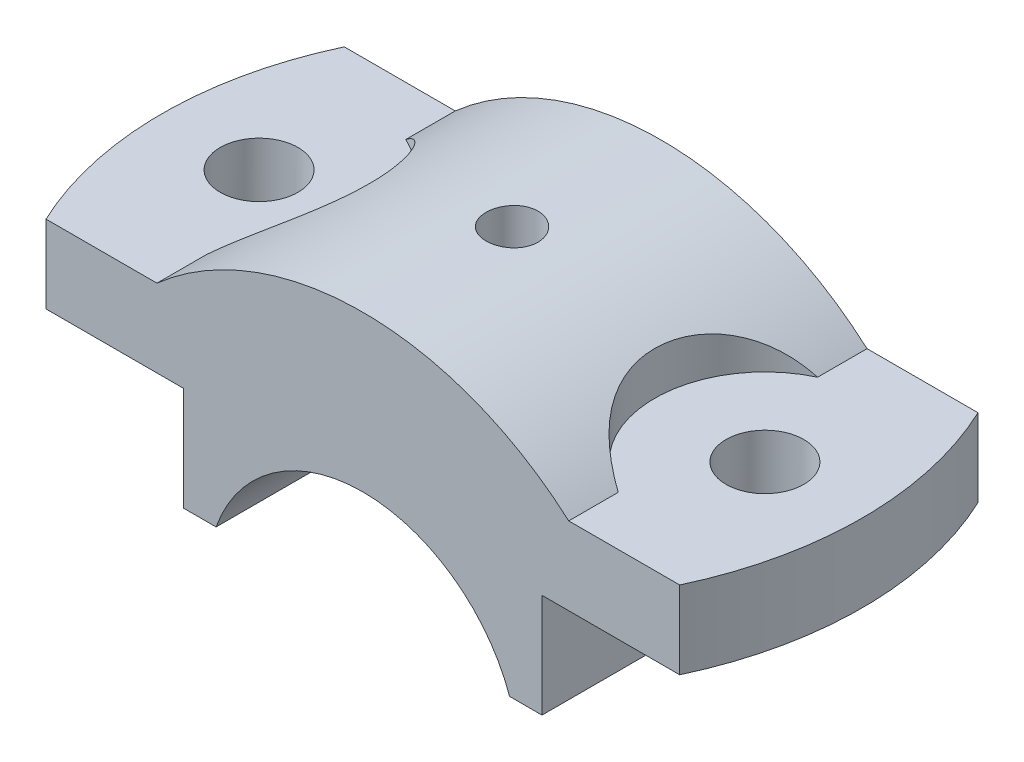
SolidWorks part; units mm, degrees
material "Plain Carbon Steel"
ref_plane "Front Plane" through (0, 0, 0) normal (0, 0, 1) x (1, 0, 0)
ref_plane "Top Plane" through (0, 0, 0) normal (0, 1, 0) x (1, 0, 0)
ref_plane "Right Plane" through (0, 0, 0) normal (1, 0, 0) x (0, 0, -1)
sketch "Cap Profile Sketch" plane through (0, 0, 0) normal (0, 0, 1) x (1, 0, 0)
  line L0 (0, 50.984) -> (0, -44.433) construction
  line L1 (-22.6274, 8) -> (-27.6274, 8)
  line L2 (-27.6274, 8) -> (-27.6274, 24)
  line L3 (-27.6274, 24) -> (-54, 24)
  line L4 (-54, 24) -> (-54, 36)
  line L5 (-54, 36) -> (-31.749, 36)
  line L6 (0, -22) -> (0, 22) construction
  line L7 (54, 36) -> (31.749, 36)
  line L8 (54, 24) -> (54, 36)
  line L9 (22.6274, 8) -> (27.6274, 8)
  line L10 (27.6274, 8) -> (27.6274, 24)
  line L11 (27.6274, 24) -> (54, 24)
  arc A0 (-22.6274, 8) -> (22.6274, 8) centre (0, 0) cw
  arc A1 (-31.749, 36) -> (31.749, 36) centre (0, 0) cw
  dimension "D1" = 24
  dimension "D2" = 48
  dimension "D3" = 8
  dimension "D4" = 16
  dimension "D5" = 5
  dimension "D6" = 12
  dimension "D7" = 54
extrude "Cap Body" add sketch "Cap Profile Sketch" along normal mid plane 46
hole_wizard "Bolt Holes Ø12" positions "Sketch2" profile "Sketch4" hole size "Ø1.0" standard "ANSI Metric" end condition through all
sketch "Sketch2" plane through (0, 36, 0) normal (0, 1, 0) x (1, 0, 0)
  point P0 (-39, 0)
  point P2 (39, 0)
  dimension "D1" = 39
  dimension "D2" = 39
sketch "Sketch4" plane through (-39, 36, 0) normal (1, 0, 0) x (0, 0, 1)
  line L0 (0, 0) -> (0, 28)
  line L1 (0, 28) -> (6, 28)
  line L2 (6, 28) -> (6, 0)
  line L5 (6, 0) -> (0, 0)
  line L11 (0, -6.35) -> (0, 107.95) construction
  dimension "Thru Hole Dia." = 12
  dimension "Thru Hole Depth" = 28
hole_wizard "Hole Ø34" positions "Sketch5" profile "Sketch7" hole size "Ø1.0" standard "ANSI Metric"
sketch "Sketch5" plane through (0, 36, 0) normal (0, 1, 0) x (1, 0, 0)
  point P0 (-39, 0)
  point P3 (39, 0)
sketch "Sketch7" plane through (-39, 36, 0) normal (1, 0, 0) x (0, 0, -1)
  line L0 (0, 0) -> (0, 36)
  line L1 (0, 36) -> (17, 36)
  line L2 (17, 36) -> (17, 0)
  line L5 (17, 0) -> (0, 0)
  line L10 (0, 36) -> (-17, 36) construction
  line L11 (0, -6.35) -> (0, 107.95) construction
  dimension "Hole Dia." = 34
  dimension "Hole Depth" = 36
  dimension "Drill Angle" = 180
ref_plane "Lube Hole Plane" through (0, 48, 0) normal (0, 1, 0) x (1, 0, 0)
sketch "Lube Counterbore Sketch Ø8" plane through (0, 48, 0) normal (0, 1, 0) x (1, 0, 0)
  circle A0 centre (0, 0) radius 4
  dimension "D1" = 8
extrude "Lube Counterbore Ø8" cut sketch "Lube Counterbore Sketch Ø8" against normal blind 16
sketch "Lube Hole Sketch Ø6" plane through (0, 48, 0) normal (0, 1, 0) x (1, 0, 0)
  circle A0 centre (0, 0) radius 3
  dimension "D1" = 6
extrude "Lube Hole Ø6" cut sketch "Lube Hole Sketch Ø6" against normal through all
sketch "Side Relief Sketch" plane through (0, 36, 0) normal (0, 1, 0) x (1, 0, 0)
  line L0 (-31.749, 23) -> (31.749, 23)
  line L1 (-31.749, -23) -> (31.749, -23)
  line L2 (0, -22) -> (0, 22) construction
  line L5 (-31.749, 23) -> (-54, 23)
  line L6 (-54, 23) -> (-54, -23)
  line L7 (-54, -23) -> (-31.749, -23)
  line L8 (-31.749, -23) -> (-31.749, -15.3761)
  line L9 (-31.749, 15.3761) -> (-31.749, 23)
  line L10 (-31.749, 23) -> (-48.8569, 23)
  line L12 (-48.8569, -23) -> (-31.749, -23)
  line L15 (31.749, 23) -> (31.749, 15.3761)
  line L16 (31.749, -15.3761) -> (31.749, -23)
  line L17 (31.749, -23) -> (54, -23)
  line L18 (54, -23) -> (54, 23)
  line L19 (54, 23) -> (31.749, 23)
  line L22 (31.749, -23) -> (48.8569, -23)
  line L24 (48.8569, 23) -> (31.749, 23)
  arc A0 (-48.8569, -23) -> (-48.8569, 23) centre (0, 0) cw
  arc A1 (-31.749, -15.3761) -> (-31.749, 15.3761) centre (-39, 0) ccw
  arc A3 (31.749, 15.3761) -> (31.749, -15.3761) centre (39, 0) ccw
  arc A5 (48.8569, -23) -> (48.8569, 23) centre (0, 0) ccw
  dimension "D3" = 54
  dimension "D1" = 0
  dimension "D2" = 0
extrude "Side Relief Cut" cut sketch "Side Relief Sketch" against normal through all flip side to cut
